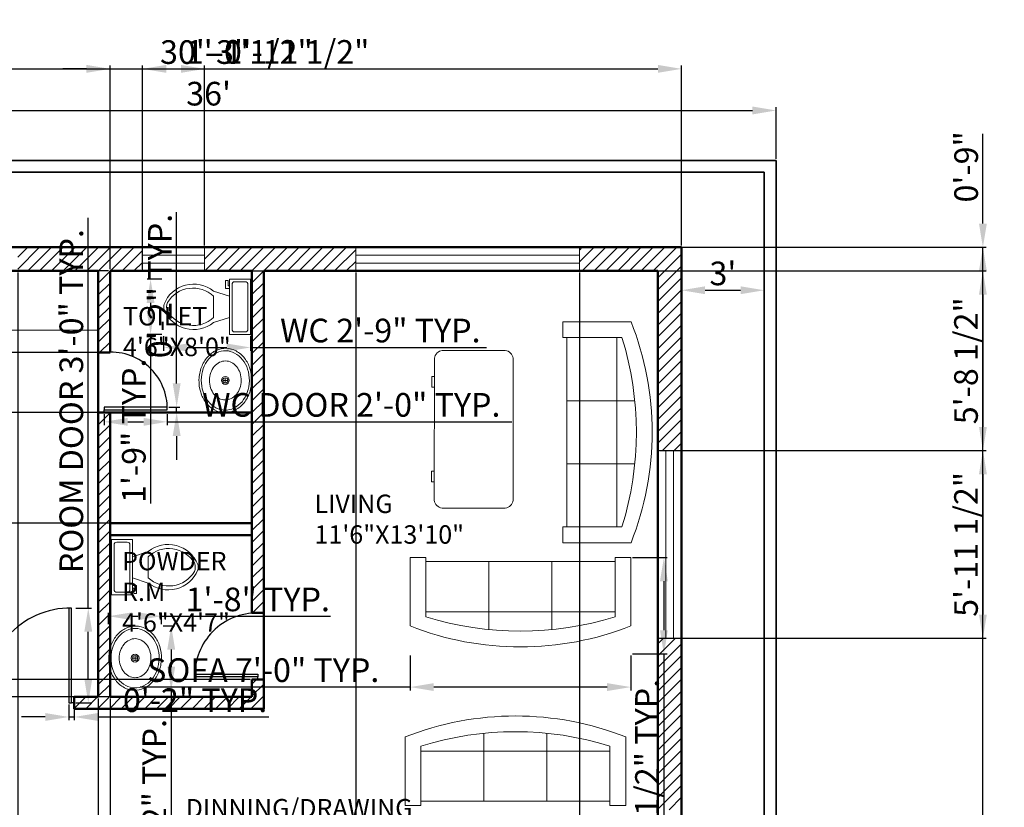
# Model space of a CAD drawing. Units: inches. Extents: x 53662 to 54269, y 37303 to 38048.
# Tile 6 of 6: x 53894 to 54269, y 37749 to 38048. Entities that reach past the tile are written whole.
import ezdxf

# ---------------------------------------------------------------- set-up
doc = ezdxf.new("R2010")
doc.units = ezdxf.units.IN
for name, color, linetype, lineweight in [('A-ANNO-DIMS', 2, 'Continuous', 18), ('A-AREA-IDEN', 7, 'Continuous', 25), ('A-DOOR', 3, 'Continuous', 25), ('A-FLOR-CASE', 8, 'Continuous', 18), ('A-FLOR-FIXT', 9, 'Continuous', 18), ('A-FURN', 8, 'Continuous', 18), ('A-GLAZ', 4, 'Continuous', 18), ('A-WALL', 7, 'Continuous', 50), ('C-PROP', 7, 'Continuous', 35)]:
    doc.layers.add(name, color=color, linetype=linetype, lineweight=lineweight)
doc.layers.add('A-WALL-PATT', color=244, linetype='Continuous', lineweight=13, true_color=0x991b1e)
doc.styles.get("Standard").update_dxf_attribs({"font": 'arial.ttf'})
doc.dimstyles.new('ISO-25', dxfattribs={"dimtxt": 9, "dimasz": 9, "dimexe": 1.25, "dimexo": 0.625, "dimtad": 1, "dimdec": 1, "dimrnd": 9, "dimlunit": 3, "dimtxsty": 'Standard', "dimcen": 2.5, "dimadec": 0, "dimazin": 0, "dimtfac": 1, "dimtdec": 1, "dimtmove": 0, "dimatfit": 3, "dimfxl": 1, "dimarcsym": 0})

# ---------------------------------------------------------------- blocks, each defined once
blk = doc.blocks.new('Toilet - top')
for p, q in [((9.5, -6), (9.5, -2)), ((-10, -8.5), (-8, -8.5)), ((-10, -9.5), (-10, -8.5)), ((-7, -9.5), (-10, -9.5)), ((-8, -8.5), (-8, -8)), ((-7, -8), (-7, -9.5)), ((-4, -8), (-6, -14)), ((4, -8), (6, -14)), ((4, -14), (-4, -14))]:
    blk.add_line(p, q)
blk.add_lwpolyline([(10.5, -8), (10.5, 0), (-10.5, 0), (-10.5, -8)], close=True)
for points in [[(-9.5, -2), (-9.5, -6)], [(8.5, -1), (-8.5, -1)], [(-8.5, -7), (8.5, -7)]]:
    blk.add_lwpolyline(points)
for centre, radius, start, end in [((-8.62, -1.88), 0.884, 81.8699, 188.1301), ((8.62, -1.88), 0.884, 351.8699, 98.1301), ((-8.62, -6.12), 0.884, 171.8699, 278.1301), ((8.62, -6.12), 0.884, 261.8699, 8.1301), ((3.52, -21.58), 12.17, 141.4691, 247.9714), ((4.2, -21.82), 11.33, 136.3677, 238.9468), ((-3.52, -21.58), 12.17, 292.0284, 38.5307), ((-4.2, -21.82), 11.33, 301.053, 43.6321), ((0, -27.88), 4, 245.7318, 294.2682), ((0, -29), 4, 254.8605, 285.1395)]:
    blk.add_arc(centre, radius, start, end)
blk = doc.blocks.new('Sink - Oval top')
for p, q in [((-1, 0), (1, 0)), ((0, 1), (0, -1))]:
    blk.add_line(p, q)
for points in [[(-12.23, 0.39, 0.117634), (-11.46, -3.36, 0.104469), (-8.88, -6.8, 0.090016), (-5.08, -9.07, 0.08192), (-0.32, -10.02, 0.08192), (4.49, -9.38, 0.090016), (8.42, -7.36, 0.104469), (11.22, -4.09, 0.117634), (12.23, -0.39, 0.117634), (11.46, 3.36, 0.104469), (8.88, 6.8, 0.090016), (5.08, 9.07, 0.08192), (0.32, 10.02, 0.08192), (-4.49, 9.38, 0.090016), (-8.42, 7.36, 0.104469), (-11.22, 4.09, 0.117634)], [(-11.29, 0.16, 0.118622), (-10.52, -3.25, 0.104678), (-8.07, -6.36, 0.089562), (-4.54, -8.37, 0.081185), (-0.13, -9.15, 0.081185), (4.3, -8.49, 0.089562), (7.89, -6.58, 0.104678), (10.42, -3.55, 0.118622), (11.29, -0.16, 0.118622), (10.52, 3.25, 0.104678), (8.07, 6.36, 0.089562), (4.54, 8.37, 0.081185), (0.13, 9.15, 0.081185), (-4.3, 8.49, 0.089562), (-7.89, 6.58, 0.104678), (-10.42, 3.55, 0.118622)], [(-7.42, 0.08, 0.118283), (-6.91, -2.17, 0.104607), (-5.29, -4.21, 0.089718), (-2.97, -5.53, 0.081436), (-0.07, -6.04, 0.081436), (2.84, -5.59, 0.089718), (5.2, -4.33, 0.104607), (6.86, -2.32, 0.118283), (7.42, -0.08, 0.118283), (6.91, 2.17, 0.104607), (5.29, 4.21, 0.089718), (2.97, 5.53, 0.081436), (0.07, 6.04, 0.081436), (-2.84, 5.59, 0.089718), (-5.2, 4.33, 0.104607), (-6.86, 2.32, 0.118283)]]:
    blk.add_lwpolyline(points, format="xyb", close=True)
for radius in [1.5, 1]:
    blk.add_circle((0, 0), radius)
blk = doc.blocks.new('Sofa - Roundback 7 ft.')
for p, q in [((-12.00002, -32.4421), (-12.00003, -6.5971)), ((11.99997, -32.4421), (11.99998, -6.5971)), ((-36.000027, -34), (-36.000027, -11.4696)), ((-35.999844, -13.3819), (35.9998, -13.3819)), ((35.99998, -34), (35.99998, -11.4696)), ((-36.000027, -32.4421), (35.99998, -32.4421))]:
    blk.add_line(p, q)
for points in [[(-36.000027, -34), (-42.000027, -34), (-42.000027, -8)], [(41.99998, -8), (41.99998, -34), (35.99998, -34)]]:
    blk.add_lwpolyline(points)
for centre, radius, start, end in [((0, -114.25), 114.25, 68.43141, 111.5686), ((-0.00001, -127.1968), 121.1968, 72.72033, 107.2797)]:
    blk.add_arc(centre, radius, start, end)
blk = doc.blocks.new('Desk - 30 x 60 in.')
for p, q in [((-26.999995, 0), (26.999995, 0)), ((-29.999995, -27), (-29.999995, -3)), ((29.999995, -3), (29.999995, -27)), ((26.999995, -30), (-26.999995, -30)), ((-20.000005, -30), (-20.000005, -31)), ((-20.000005, -31), (-16.000005, -31)), ((-16.000005, -31), (-16.000005, -30)), ((15.999995, -31), (15.999995, -30)), ((19.999995, -31), (15.999995, -31)), ((19.999995, -30), (19.999995, -31))]:
    blk.add_line(p, q)
for centre, start, end in [((-26.499995, -3.5), 98.1301, 171.8699), ((26.499995, -3.5), 8.130102, 81.8699), ((-26.499995, -26.5), 188.1301, 261.8699), ((26.499995, -26.5), 278.1301, 351.8699)]:
    blk.add_arc(centre, 3.535534, start, end)
blk = doc.blocks.new('*D11')
at = {"layer": 'A-ANNO-DIMS', "color": 0, "lineweight": -2, "transparency": 16777216}
for p, q in [((54146.11, 37961.24), (54146.11, 37944.26)), ((54177.61, 37961.24), (54177.61, 37944.26)), ((54155.11, 37945.51), (54168.61, 37945.51))]:
    blk.add_line(p, q, dxfattribs=at)
at = {"layer": 'A-ANNO-DIMS', "color": 0, "transparency": 16777216}
for points in [[(54155.11, 37947.01), (54155.11, 37944.01), (54146.11, 37945.51)], [(54168.61, 37947.01), (54168.61, 37944.01), (54177.61, 37945.51)]]:
    blk.add_solid(points, dxfattribs=at)
at = {"layer": 'Defpoints', "color": 0, "transparency": 16777216}
for p in [(54146.11, 37961.86), (54177.61, 37961.86), (54177.61, 37945.51)]:
    blk.add_point(p, dxfattribs=at)
at = {"layer": 'A-ANNO-DIMS', "color": 0, "transparency": 16777216, "insert": (54161.86, 37950.74), "char_height": 9, "attachment_point": 5}
blk.add_mtext("3'", dxfattribs=at)
blk = doc.blocks.new('*D14')
at = {"layer": 'A-ANNO-DIMS', "color": 0, "lineweight": -2, "transparency": 16777216}
for p, q in [((53750.11, 37995.49), (53750.11, 38015.14)), ((54182.11, 37995.49), (54182.11, 38015.14)), ((53759.11, 38013.89), (54173.11, 38013.89))]:
    blk.add_line(p, q, dxfattribs=at)
at = {"layer": 'A-ANNO-DIMS', "color": 0, "transparency": 16777216}
for points in [[(53759.11, 38015.39), (53759.11, 38012.39), (53750.11, 38013.89)], [(54173.11, 38015.39), (54173.11, 38012.39), (54182.11, 38013.89)]]:
    blk.add_solid(points, dxfattribs=at)
at = {"layer": 'Defpoints', "color": 0, "transparency": 16777216}
for p in [(54182.11, 38013.89), (53750.11, 37994.86), (54182.11, 37994.86)]:
    blk.add_point(p, dxfattribs=at)
at = {"layer": 'A-ANNO-DIMS', "color": 0, "transparency": 16777216, "insert": (53966.11, 38019.11), "char_height": 9, "attachment_point": 5}
blk.add_mtext("36'", dxfattribs=at)
blk = doc.blocks.new('DOOR-LEAF-36IN')
for p, q in [((1, 36), (0, 36)), ((0, 36), (0, 0)), ((1, 0), (1, 36)), ((0, 0), (1, 0)), ((2, 0), (1, 0))]:
    blk.add_line(p, q)
blk = doc.blocks.new('DOOR-LEAF-24IN')
for p, q in [((24, 2), (0, 2)), ((0, 2), (0, 1)), ((0, 0), (0, 1)), ((0, 1), (24, 1)), ((24, 1), (24, 2))]:
    blk.add_line(p, q)
blk = doc.blocks.new('*D30')
at = {"layer": 'A-ANNO-DIMS', "color": 0, "lineweight": -2, "transparency": 16777216}
for p, q in [((54042.81, 37806.54), (54042.81, 37793.32)), ((54126.81, 37806.54), (54126.81, 37793.32)), ((54042.81, 37794.57), (53940.02, 37794.57)), ((54117.81, 37794.57), (54051.81, 37794.57))]:
    blk.add_line(p, q, dxfattribs=at)
at = {"layer": 'A-ANNO-DIMS', "color": 0, "transparency": 16777216}
for points in [[(54051.81, 37796.07), (54051.81, 37793.07), (54042.81, 37794.57)], [(54117.81, 37796.07), (54117.81, 37793.07), (54126.81, 37794.57)]]:
    blk.add_solid(points, dxfattribs=at)
at = {"layer": 'Defpoints', "color": 0, "transparency": 16777216}
for p in [(54042.81, 37807.17), (54126.81, 37807.17), (54042.81, 37794.57)]:
    blk.add_point(p, dxfattribs=at)
at = {"layer": 'A-ANNO-DIMS', "color": 0, "transparency": 16777216, "insert": (53986.91, 37799.85), "char_height": 9, "attachment_point": 5}
blk.add_mtext('SOFA 7\'-0" TYP.', dxfattribs=at)
blk = doc.blocks.new('*D31')
at = {"layer": 'A-ANNO-DIMS', "color": 0, "lineweight": -2, "transparency": 16777216}
for p, q in [((54127.43, 37843.84), (54140.66, 37843.84)), ((54139.41, 37834.84), (54139.41, 37816.17)), ((54127.43, 37807.17), (54140.66, 37807.17)), ((54139.41, 37807.17), (54139.41, 37721.1))]:
    blk.add_line(p, q, dxfattribs=at)
at = {"layer": 'A-ANNO-DIMS', "color": 0, "transparency": 16777216}
for points in [[(54137.91, 37834.84), (54140.91, 37834.84), (54139.41, 37843.84)], [(54137.91, 37816.17), (54140.91, 37816.17), (54139.41, 37807.17)]]:
    blk.add_solid(points, dxfattribs=at)
at = {"layer": 'Defpoints', "color": 0, "transparency": 16777216}
for p in [(54126.81, 37843.84), (54126.81, 37807.17), (54139.41, 37807.17)]:
    blk.add_point(p, dxfattribs=at)
at = {"layer": 'A-ANNO-DIMS', "color": 0, "transparency": 16777216, "insert": (54134.13, 37759.63), "char_height": 9, "attachment_point": 5, "rotation": 90}
blk.add_mtext('3\'-0 1/2" TYP.', dxfattribs=at)
blk = doc.blocks.new('*D36')
at = {"layer": 'A-ANNO-DIMS', "color": 0, "lineweight": -2, "transparency": 16777216}
for p, q in [((53948.99, 37928.07), (53948.99, 37922.49)), ((53982.03, 37928.07), (53982.03, 37922.49)), ((53957.99, 37923.74), (53973.03, 37923.74)), ((53982.03, 37923.74), (54071.95, 37923.74))]:
    blk.add_line(p, q, dxfattribs=at)
at = {"layer": 'A-ANNO-DIMS', "color": 0, "transparency": 16777216}
for points in [[(53957.99, 37925.24), (53957.99, 37922.24), (53948.99, 37923.74)], [(53973.03, 37925.24), (53973.03, 37922.24), (53982.03, 37923.74)]]:
    blk.add_solid(points, dxfattribs=at)
at = {"layer": 'Defpoints', "color": 0, "transparency": 16777216}
for p in [(53948.99, 37928.7), (53982.03, 37928.7), (53982.03, 37923.74)]:
    blk.add_point(p, dxfattribs=at)
at = {"layer": 'A-ANNO-DIMS', "color": 0, "transparency": 16777216, "insert": (54031.49, 37929.02), "char_height": 9, "attachment_point": 5}
blk.add_mtext('WC 2\'-9" TYP.', dxfattribs=at)
blk = doc.blocks.new('*D37')
at = {"layer": 'A-ANNO-DIMS', "color": 0, "lineweight": -2, "transparency": 16777216}
for p, q in [((53948.36, 37949.7), (53942.78, 37949.7)), ((53944.03, 37940.7), (53944.03, 37937.7)), ((53948.36, 37928.7), (53942.78, 37928.7)), ((53944.03, 37928.7), (53944.03, 37864.43))]:
    blk.add_line(p, q, dxfattribs=at)
at = {"layer": 'A-ANNO-DIMS', "color": 0, "transparency": 16777216}
for points in [[(53942.53, 37940.7), (53945.53, 37940.7), (53944.03, 37949.7)], [(53942.53, 37937.7), (53945.53, 37937.7), (53944.03, 37928.7)]]:
    blk.add_solid(points, dxfattribs=at)
at = {"layer": 'Defpoints', "color": 0, "transparency": 16777216}
for p in [(53948.99, 37949.7), (53944.03, 37928.7), (53948.99, 37928.7)]:
    blk.add_point(p, dxfattribs=at)
at = {"layer": 'A-ANNO-DIMS', "color": 0, "transparency": 16777216, "insert": (53938.81, 37892.06), "char_height": 9, "attachment_point": 5, "rotation": 90}
blk.add_mtext('1\'-9" TYP.', dxfattribs=at)
blk = doc.blocks.new('*D38')
at = {"layer": 'A-ANNO-DIMS', "color": 0, "lineweight": -2, "transparency": 16777216}
for p, q in [((53948.84, 37817.85), (53953.14, 37817.85)), ((53951.89, 37808.85), (53951.89, 37802.3)), ((53948.84, 37793.3), (53953.14, 37793.3)), ((53951.89, 37793.3), (53951.89, 37666.39))]:
    blk.add_line(p, q, dxfattribs=at)
at = {"layer": 'A-ANNO-DIMS', "color": 0, "transparency": 16777216}
for points in [[(53950.39, 37808.85), (53953.39, 37808.85), (53951.89, 37817.85)], [(53950.39, 37802.3), (53953.39, 37802.3), (53951.89, 37793.3)]]:
    blk.add_solid(points, dxfattribs=at)
at = {"layer": 'Defpoints', "color": 0, "transparency": 16777216}
for p in [(53948.21, 37817.85), (53948.21, 37793.3), (53951.89, 37793.3)]:
    blk.add_point(p, dxfattribs=at)
at = {"layer": 'A-ANNO-DIMS', "color": 0, "transparency": 16777216, "insert": (53946.62, 37725.34), "char_height": 9, "attachment_point": 5, "rotation": 90}
blk.add_mtext('BASIN 2\'-0 1/2" TYP.', dxfattribs=at)
blk = doc.blocks.new('*D39')
at = {"layer": 'A-ANNO-DIMS', "color": 0, "lineweight": -2, "transparency": 16777216}
for p, q in [((53928.07, 37818.47), (53928.07, 37822.78)), ((53937.07, 37821.53), (53939.21, 37821.53)), ((53948.21, 37818.47), (53948.21, 37822.78)), ((53948.21, 37821.53), (54012.47, 37821.53))]:
    blk.add_line(p, q, dxfattribs=at)
at = {"layer": 'A-ANNO-DIMS', "color": 0, "transparency": 16777216}
for points in [[(53937.07, 37823.03), (53937.07, 37820.03), (53928.07, 37821.53)], [(53939.21, 37823.03), (53939.21, 37820.03), (53948.21, 37821.53)]]:
    blk.add_solid(points, dxfattribs=at)
at = {"layer": 'Defpoints', "color": 0, "transparency": 16777216}
for p in [(53948.21, 37821.53), (53928.07, 37817.85), (53948.21, 37817.85)]:
    blk.add_point(p, dxfattribs=at)
at = {"layer": 'A-ANNO-DIMS', "color": 0, "transparency": 16777216, "insert": (53984.84, 37826.75), "char_height": 9, "attachment_point": 5}
blk.add_mtext('1\'-8" TYP.', dxfattribs=at)
blk = doc.blocks.new('*D40')
at = {"layer": 'A-ANNO-DIMS', "color": 0, "lineweight": -2, "transparency": 16777216}
for p, q in [((53920.32, 37824.61), (53920.32, 37973.07)), ((53915.54, 37824.61), (53921.57, 37824.61)), ((53920.32, 37797.61), (53920.32, 37815.61)), ((53915.54, 37788.61), (53921.57, 37788.61))]:
    blk.add_line(p, q, dxfattribs=at)
at = {"layer": 'A-ANNO-DIMS', "color": 0, "transparency": 16777216}
for points in [[(53918.82, 37815.61), (53921.82, 37815.61), (53920.32, 37824.61)], [(53918.82, 37797.61), (53921.82, 37797.61), (53920.32, 37788.61)]]:
    blk.add_solid(points, dxfattribs=at)
at = {"layer": 'Defpoints', "color": 0, "transparency": 16777216}
for p in [(53914.92, 37824.61), (53920.32, 37824.61), (53914.92, 37788.61)]:
    blk.add_point(p, dxfattribs=at)
at = {"layer": 'A-ANNO-DIMS', "color": 0, "transparency": 16777216, "insert": (53915.03, 37903.34), "char_height": 9, "attachment_point": 5, "rotation": 90}
blk.add_mtext('ROOM DOOR 3\'-0" TYP.', dxfattribs=at)
blk = doc.blocks.new('*D41')
at = {"layer": 'A-ANNO-DIMS', "color": 0, "lineweight": -2, "transparency": 16777216}
for p, q in [((53912.92, 37787.99), (53912.92, 37781.96)), ((53914.92, 37787.99), (53914.92, 37781.96)), ((53903.92, 37783.21), (53894.92, 37783.21)), ((53912.92, 37783.21), (53914.92, 37783.21)), ((53923.92, 37783.21), (53989.03, 37783.21))]:
    blk.add_line(p, q, dxfattribs=at)
at = {"layer": 'A-ANNO-DIMS', "color": 0, "transparency": 16777216}
for points in [[(53903.92, 37784.71), (53903.92, 37781.71), (53912.92, 37783.21)], [(53923.92, 37784.71), (53923.92, 37781.71), (53914.92, 37783.21)]]:
    blk.add_solid(points, dxfattribs=at)
at = {"layer": 'Defpoints', "color": 0, "transparency": 16777216}
for p in [(53912.92, 37788.61), (53914.92, 37788.61), (53914.92, 37783.21)]:
    blk.add_point(p, dxfattribs=at)
at = {"layer": 'A-ANNO-DIMS', "color": 0, "transparency": 16777216, "insert": (53960.97, 37788.43), "char_height": 9, "attachment_point": 5}
blk.add_mtext('0\'-2" TYP.', dxfattribs=at)
blk = doc.blocks.new('*D42')
at = {"layer": 'A-ANNO-DIMS', "color": 0, "lineweight": -2, "transparency": 16777216}
for p, q in [((53926.36, 37898.44), (53926.36, 37894.21)), ((53950.36, 37898.44), (53950.36, 37894.21)), ((53935.36, 37895.46), (53941.36, 37895.46)), ((53950.36, 37895.46), (54081.49, 37895.46))]:
    blk.add_line(p, q, dxfattribs=at)
at = {"layer": 'A-ANNO-DIMS', "color": 0, "transparency": 16777216}
for points in [[(53935.36, 37896.96), (53935.36, 37893.96), (53926.36, 37895.46)], [(53941.36, 37896.96), (53941.36, 37893.96), (53950.36, 37895.46)]]:
    blk.add_solid(points, dxfattribs=at)
at = {"layer": 'Defpoints', "color": 0, "transparency": 16777216}
for p in [(53926.36, 37899.06), (53950.36, 37899.06), (53950.36, 37895.46)]:
    blk.add_point(p, dxfattribs=at)
at = {"layer": 'A-ANNO-DIMS', "color": 0, "transparency": 16777216, "insert": (54020.43, 37900.75), "char_height": 9, "attachment_point": 5}
blk.add_mtext('WC DOOR 2\'-0" TYP.', dxfattribs=at)
blk = doc.blocks.new('*D43')
at = {"layer": 'A-ANNO-DIMS', "color": 0, "lineweight": -2, "transparency": 16777216}
for p, q in [((53953.96, 37910.06), (53953.96, 37975.17)), ((53950.99, 37901.06), (53955.21, 37901.06)), ((53950.99, 37899.06), (53955.21, 37899.06)), ((53953.96, 37899.06), (53953.96, 37901.06)), ((53953.96, 37890.06), (53953.96, 37881.06))]:
    blk.add_line(p, q, dxfattribs=at)
at = {"layer": 'A-ANNO-DIMS', "color": 0, "transparency": 16777216}
for points in [[(53952.46, 37910.06), (53955.46, 37910.06), (53953.96, 37901.06)], [(53952.46, 37890.06), (53955.46, 37890.06), (53953.96, 37899.06)]]:
    blk.add_solid(points, dxfattribs=at)
at = {"layer": 'Defpoints', "color": 0, "transparency": 16777216}
for p in [(53950.36, 37901.06), (53950.36, 37899.06), (53953.96, 37901.06)]:
    blk.add_point(p, dxfattribs=at)
at = {"layer": 'A-ANNO-DIMS', "color": 0, "transparency": 16777216, "insert": (53948.74, 37947.12), "char_height": 9, "attachment_point": 5, "rotation": 90}
blk.add_mtext('0\'-2" TYP.', dxfattribs=at)
blk = doc.blocks.new('*D50')
at = {"layer": 'A-ANNO-DIMS', "color": 0, "lineweight": -2, "transparency": 16777216}
for p, q in [((53783.11, 37962.49), (53783.11, 38030.96)), ((53792.11, 38029.71), (54137.11, 38029.71)), ((54146.11, 37962.49), (54146.11, 38030.96))]:
    blk.add_line(p, q, dxfattribs=at)
at = {"layer": 'A-ANNO-DIMS', "color": 0, "transparency": 16777216}
for points in [[(53792.11, 38031.21), (53792.11, 38028.21), (53783.11, 38029.71)], [(54137.11, 38031.21), (54137.11, 38028.21), (54146.11, 38029.71)]]:
    blk.add_solid(points, dxfattribs=at)
at = {"layer": 'Defpoints', "color": 0, "transparency": 16777216}
for p in [(54146.11, 38029.71), (53783.11, 37961.86), (54146.11, 37961.86)]:
    blk.add_point(p, dxfattribs=at)
at = {"layer": 'A-ANNO-DIMS', "color": 0, "transparency": 16777216, "insert": (53964.61, 38034.93), "char_height": 9, "attachment_point": 5}
blk.add_mtext('30\'-3"', dxfattribs=at)
blk = doc.blocks.new('*D51')
at = {"layer": 'A-ANNO-DIMS', "color": 0, "lineweight": -2, "transparency": 16777216}
for p, q in [((54146.74, 37961.86), (54262.07, 37961.86)), ((54260.82, 37471.86), (54260.82, 37952.86)), ((53987.74, 37462.86), (54262.07, 37462.86))]:
    blk.add_line(p, q, dxfattribs=at)
at = {"layer": 'A-ANNO-DIMS', "color": 0, "transparency": 16777216}
for points in [[(54259.32, 37952.86), (54262.32, 37952.86), (54260.82, 37961.86)], [(54259.32, 37471.86), (54262.32, 37471.86), (54260.82, 37462.86)]]:
    blk.add_solid(points, dxfattribs=at)
at = {"layer": 'Defpoints', "color": 0, "transparency": 16777216}
for p in [(54146.11, 37961.86), (54260.82, 37961.86), (53987.11, 37462.86)]:
    blk.add_point(p, dxfattribs=at)
at = {"layer": 'A-ANNO-DIMS', "color": 0, "transparency": 16777216, "insert": (54255.68, 37712.36), "char_height": 9, "attachment_point": 5, "rotation": 90}
blk.add_mtext('41\'-7"', dxfattribs=at)
blk = doc.blocks.new('*D55')
at = {"layer": 'A-ANNO-DIMS', "color": 0, "lineweight": -2, "transparency": 16777216}
for p, q in [((53849.2, 37952.24), (53849.2, 37309.49)), ((53893.52, 37952.24), (53893.52, 37309.49)), ((53858.2, 37310.74), (53884.52, 37310.74)), ((53893.52, 37310.74), (53948.66, 37310.74))]:
    blk.add_line(p, q, dxfattribs=at)
at = {"layer": 'A-ANNO-DIMS', "color": 0, "transparency": 16777216}
for points in [[(53858.2, 37312.24), (53858.2, 37309.24), (53849.2, 37310.74)], [(53884.52, 37312.24), (53884.52, 37309.24), (53893.52, 37310.74)]]:
    blk.add_solid(points, dxfattribs=at)
at = {"layer": 'Defpoints', "color": 0, "transparency": 16777216}
for p in [(53849.2, 37952.86), (53893.52, 37952.86), (53893.52, 37310.74)]:
    blk.add_point(p, dxfattribs=at)
at = {"layer": 'A-ANNO-DIMS', "color": 0, "transparency": 16777216, "insert": (53925.59, 37316.02), "char_height": 9, "attachment_point": 5}
blk.add_mtext('3\'-8 1/2"', dxfattribs=at)
blk = doc.blocks.new('*D56')
at = {"layer": 'A-ANNO-DIMS', "color": 0, "lineweight": -2, "transparency": 16777216}
for p, q in [((53919.61, 38029.71), (53910.61, 38029.71)), ((53928.61, 37953.49), (53928.61, 38030.96)), ((53928.61, 38029.71), (53940.97, 38029.71)), ((53940.97, 37953.49), (53940.97, 38030.96)), ((53949.97, 38029.71), (54004.27, 38029.71))]:
    blk.add_line(p, q, dxfattribs=at)
at = {"layer": 'A-ANNO-DIMS', "color": 0, "transparency": 16777216}
for points in [[(53919.61, 38031.21), (53919.61, 38028.21), (53928.61, 38029.71)], [(53949.97, 38031.21), (53949.97, 38028.21), (53940.97, 38029.71)]]:
    blk.add_solid(points, dxfattribs=at)
at = {"layer": 'Defpoints', "color": 0, "transparency": 16777216}
for p in [(53940.97, 38029.71), (53928.61, 37952.86), (53940.97, 37952.86)]:
    blk.add_point(p, dxfattribs=at)
at = {"layer": 'A-ANNO-DIMS', "color": 0, "transparency": 16777216, "insert": (53981.62, 38034.99), "char_height": 9, "attachment_point": 5}
blk.add_mtext('1\'-0 1/2"', dxfattribs=at)
blk = doc.blocks.new('*D57')
at = {"layer": 'A-ANNO-DIMS', "color": 0, "lineweight": -2, "transparency": 16777216}
for p, q in [((53940.97, 37962.49), (53940.97, 38030.96)), ((53949.97, 38029.71), (53955.61, 38029.71)), ((53964.61, 37962.49), (53964.61, 38030.96)), ((53964.61, 38029.71), (54025.91, 38029.71))]:
    blk.add_line(p, q, dxfattribs=at)
at = {"layer": 'A-ANNO-DIMS', "color": 0, "transparency": 16777216}
for points in [[(53949.97, 38031.21), (53949.97, 38028.21), (53940.97, 38029.71)], [(53955.61, 38031.21), (53955.61, 38028.21), (53964.61, 38029.71)]]:
    blk.add_solid(points, dxfattribs=at)
at = {"layer": 'Defpoints', "color": 0, "transparency": 16777216}
for p in [(53964.61, 38029.71), (53940.97, 37961.86), (53964.61, 37961.86)]:
    blk.add_point(p, dxfattribs=at)
at = {"layer": 'A-ANNO-DIMS', "color": 0, "transparency": 16777216, "insert": (53999.76, 38034.99), "char_height": 9, "attachment_point": 5}
blk.add_mtext('1\'-11 1/2"', dxfattribs=at)
blk = doc.blocks.new('*D58')
at = {"layer": 'A-ANNO-DIMS', "color": 0, "lineweight": -2, "transparency": 16777216}
for p, q in [((54022.12, 37952.24), (54022.12, 37309.49)), ((54107.27, 37952.24), (54107.27, 37309.49)), ((54031.12, 37310.74), (54098.27, 37310.74))]:
    blk.add_line(p, q, dxfattribs=at)
at = {"layer": 'A-ANNO-DIMS', "color": 0, "transparency": 16777216}
for points in [[(54031.12, 37312.24), (54031.12, 37309.24), (54022.12, 37310.74)], [(54098.27, 37312.24), (54098.27, 37309.24), (54107.27, 37310.74)]]:
    blk.add_solid(points, dxfattribs=at)
at = {"layer": 'Defpoints', "color": 0, "transparency": 16777216}
for p in [(54022.12, 37952.86), (54107.27, 37952.86), (54107.27, 37310.74)]:
    blk.add_point(p, dxfattribs=at)
at = {"layer": 'A-ANNO-DIMS', "color": 0, "transparency": 16777216, "insert": (54064.7, 37315.88), "char_height": 9, "attachment_point": 5}
blk.add_mtext('7\'-1"', dxfattribs=at)
blk = doc.blocks.new('*D59')
at = {"layer": 'A-ANNO-DIMS', "color": 0, "lineweight": -2, "transparency": 16777216}
for p, q in [((54107.27, 37952.24), (54107.27, 37309.49)), ((54137.11, 37952.24), (54137.11, 37309.49)), ((54116.27, 37310.74), (54128.11, 37310.74))]:
    blk.add_line(p, q, dxfattribs=at)
at = {"layer": 'A-ANNO-DIMS', "color": 0, "transparency": 16777216}
for points in [[(54116.27, 37312.24), (54116.27, 37309.24), (54107.27, 37310.74)], [(54128.11, 37312.24), (54128.11, 37309.24), (54137.11, 37310.74)]]:
    blk.add_solid(points, dxfattribs=at)
at = {"layer": 'Defpoints', "color": 0, "transparency": 16777216}
for p in [(54107.27, 37952.86), (54137.11, 37952.86), (54137.11, 37310.74)]:
    blk.add_point(p, dxfattribs=at)
at = {"layer": 'A-ANNO-DIMS', "color": 0, "transparency": 16777216, "insert": (54122.19, 37315.96), "char_height": 9, "attachment_point": 5}
blk.add_mtext('2\'-6"', dxfattribs=at)
blk = doc.blocks.new('*D60')
at = {"layer": 'A-ANNO-DIMS', "color": 0, "lineweight": -2, "transparency": 16777216}
for p, q in [((53924.11, 37790.24), (53924.11, 37309.49)), ((53928.61, 37790.24), (53928.61, 37309.49)), ((53915.11, 37310.74), (53906.11, 37310.74)), ((53924.11, 37310.74), (53928.61, 37310.74)), ((53937.61, 37310.74), (53992.76, 37310.74))]:
    blk.add_line(p, q, dxfattribs=at)
at = {"layer": 'A-ANNO-DIMS', "color": 0, "transparency": 16777216}
for points in [[(53915.11, 37312.24), (53915.11, 37309.24), (53924.11, 37310.74)], [(53937.61, 37312.24), (53937.61, 37309.24), (53928.61, 37310.74)]]:
    blk.add_solid(points, dxfattribs=at)
at = {"layer": 'Defpoints', "color": 0, "transparency": 16777216}
for p in [(53924.11, 37790.86), (53928.61, 37790.86), (53928.61, 37310.74)]:
    blk.add_point(p, dxfattribs=at)
at = {"layer": 'A-ANNO-DIMS', "color": 0, "transparency": 16777216, "insert": (53969.69, 37316.02), "char_height": 9, "attachment_point": 5}
blk.add_mtext('0\'-4 1/2"', dxfattribs=at)
blk = doc.blocks.new('*D61')
at = {"layer": 'A-ANNO-DIMS', "color": 0, "lineweight": -2, "transparency": 16777216}
for p, q in [((54260.82, 37970.86), (54260.82, 38005.03)), ((53965.24, 37961.86), (54262.07, 37961.86)), ((54260.82, 37952.86), (54260.82, 37961.86)), ((53965.24, 37952.86), (54262.07, 37952.86)), ((54260.82, 37943.86), (54260.82, 37934.86))]:
    blk.add_line(p, q, dxfattribs=at)
at = {"layer": 'A-ANNO-DIMS', "color": 0, "transparency": 16777216}
for points in [[(54259.32, 37970.86), (54262.32, 37970.86), (54260.82, 37961.86)], [(54259.32, 37943.86), (54262.32, 37943.86), (54260.82, 37952.86)]]:
    blk.add_solid(points, dxfattribs=at)
at = {"layer": 'Defpoints', "color": 0, "transparency": 16777216}
for p in [(53964.61, 37961.86), (54260.82, 37961.86), (53964.61, 37952.86)]:
    blk.add_point(p, dxfattribs=at)
at = {"layer": 'A-ANNO-DIMS', "color": 0, "transparency": 16777216, "insert": (54255.6, 37992.45), "char_height": 9, "attachment_point": 5, "rotation": 90}
blk.add_mtext('0\'-9"', dxfattribs=at)
blk = doc.blocks.new('*D66')
at = {"layer": 'A-ANNO-DIMS', "color": 0, "lineweight": -2, "transparency": 16777216}
for p, q in [((54137.74, 37952.86), (54262.07, 37952.86)), ((54260.82, 37943.86), (54260.82, 37893.55)), ((54137.74, 37884.55), (54262.07, 37884.55))]:
    blk.add_line(p, q, dxfattribs=at)
at = {"layer": 'A-ANNO-DIMS', "color": 0, "transparency": 16777216}
for points in [[(54259.32, 37943.86), (54262.32, 37943.86), (54260.82, 37952.86)], [(54259.32, 37893.55), (54262.32, 37893.55), (54260.82, 37884.55)]]:
    blk.add_solid(points, dxfattribs=at)
at = {"layer": 'Defpoints', "color": 0, "transparency": 16777216}
for p in [(54137.11, 37952.86), (54137.11, 37884.55), (54260.82, 37884.55)]:
    blk.add_point(p, dxfattribs=at)
at = {"layer": 'A-ANNO-DIMS', "color": 0, "transparency": 16777216, "insert": (54255.55, 37918.7), "char_height": 9, "attachment_point": 5, "rotation": 90}
blk.add_mtext('5\'-8 1/2"', dxfattribs=at)
blk = doc.blocks.new('*D67')
at = {"layer": 'A-ANNO-DIMS', "color": 0, "lineweight": -2, "transparency": 16777216}
for p, q in [((54137.74, 37884.55), (54262.07, 37884.55)), ((54260.82, 37875.55), (54260.82, 37822.18)), ((54137.74, 37813.18), (54262.07, 37813.18))]:
    blk.add_line(p, q, dxfattribs=at)
at = {"layer": 'A-ANNO-DIMS', "color": 0, "transparency": 16777216}
for points in [[(54259.32, 37875.55), (54262.32, 37875.55), (54260.82, 37884.55)], [(54259.32, 37822.18), (54262.32, 37822.18), (54260.82, 37813.18)]]:
    blk.add_solid(points, dxfattribs=at)
at = {"layer": 'Defpoints', "color": 0, "transparency": 16777216}
for p in [(54137.11, 37884.55), (54137.11, 37813.18), (54260.82, 37813.18)]:
    blk.add_point(p, dxfattribs=at)
at = {"layer": 'A-ANNO-DIMS', "color": 0, "transparency": 16777216, "insert": (54255.55, 37848.86), "char_height": 9, "attachment_point": 5, "rotation": 90}
blk.add_mtext('5\'-11 1/2"', dxfattribs=at)
blk = doc.blocks.new('*D72')
at = {"layer": 'A-ANNO-DIMS', "color": 0, "lineweight": -2, "transparency": 16777216}
for p, q in [((53981.99, 37899.06), (53679.5, 37899.06)), ((53680.75, 37865.86), (53680.75, 37890.06)), ((53981.99, 37856.86), (53679.5, 37856.86))]:
    blk.add_line(p, q, dxfattribs=at)
at = {"layer": 'A-ANNO-DIMS', "color": 0, "transparency": 16777216}
for points in [[(53679.25, 37890.06), (53682.25, 37890.06), (53680.75, 37899.06)], [(53679.25, 37865.86), (53682.25, 37865.86), (53680.75, 37856.86)]]:
    blk.add_solid(points, dxfattribs=at)
at = {"layer": 'Defpoints', "color": 0, "transparency": 16777216}
for p in [(53680.75, 37899.06), (53982.61, 37899.06), (53982.61, 37856.86)]:
    blk.add_point(p, dxfattribs=at)
at = {"layer": 'A-ANNO-DIMS', "color": 0, "transparency": 16777216, "insert": (53675.53, 37877.96), "char_height": 9, "attachment_point": 5, "rotation": 90}
blk.add_mtext('3\'-6"', dxfattribs=at)
blk = doc.blocks.new('*D73')
at = {"layer": 'A-ANNO-DIMS', "color": 0, "lineweight": -2, "transparency": 16777216}
for p, q in [((53927.99, 37952.86), (53679.5, 37952.86)), ((53680.75, 37930.83), (53680.75, 37943.86)), ((53927.99, 37921.83), (53679.5, 37921.83))]:
    blk.add_line(p, q, dxfattribs=at)
at = {"layer": 'A-ANNO-DIMS', "color": 0, "transparency": 16777216}
for points in [[(53679.25, 37943.86), (53682.25, 37943.86), (53680.75, 37952.86)], [(53679.25, 37930.83), (53682.25, 37930.83), (53680.75, 37921.83)]]:
    blk.add_solid(points, dxfattribs=at)
at = {"layer": 'Defpoints', "color": 0, "transparency": 16777216}
for p in [(53680.75, 37952.86), (53928.61, 37952.86), (53928.61, 37921.83)]:
    blk.add_point(p, dxfattribs=at)
at = {"layer": 'A-ANNO-DIMS', "color": 0, "transparency": 16777216, "insert": (53675.61, 37937.35), "char_height": 9, "attachment_point": 5, "rotation": 90}
blk.add_mtext('2\'-7"', dxfattribs=at)
blk = doc.blocks.new('*D74')
at = {"layer": 'A-ANNO-DIMS', "color": 0, "lineweight": -2, "transparency": 16777216}
for p, q in [((53680.75, 37806.48), (53680.75, 37861.62)), ((53981.99, 37797.48), (53679.5, 37797.48)), ((53680.75, 37790.86), (53680.75, 37797.48)), ((53981.99, 37790.86), (53679.5, 37790.86)), ((53680.75, 37781.86), (53680.75, 37772.86))]:
    blk.add_line(p, q, dxfattribs=at)
at = {"layer": 'A-ANNO-DIMS', "color": 0, "transparency": 16777216}
for points in [[(53679.25, 37806.48), (53682.25, 37806.48), (53680.75, 37797.48)], [(53679.25, 37781.86), (53682.25, 37781.86), (53680.75, 37790.86)]]:
    blk.add_solid(points, dxfattribs=at)
at = {"layer": 'Defpoints', "color": 0, "transparency": 16777216}
for p in [(53680.75, 37797.48), (53982.61, 37797.48), (53982.61, 37790.86)]:
    blk.add_point(p, dxfattribs=at)
at = {"layer": 'A-ANNO-DIMS', "color": 0, "transparency": 16777216, "insert": (53675.47, 37838.55), "char_height": 9, "attachment_point": 5, "rotation": 90}
blk.add_mtext('0\'-6 1/2"', dxfattribs=at)

msp = doc.modelspace()

# ---------------------------------------------------------------- hatches: boundary and pattern name
at = {"layer": 'A-WALL-PATT'}
h = msp.add_hatch(dxfattribs=at)
h.set_pattern_fill('ANSI31', color=256)
h.paths.add_polyline_path([(53792.11, 37952.86), (53849.2, 37952.86), (53849.2, 37961.86), (53783.11, 37961.86), (53783.11, 37861.42), (53792.11, 37861.42)])
h.paths.add_polyline_path([(53940.97, 37961.86), (53893.52, 37961.86), (53893.52, 37952.86), (53924.11, 37952.86), (53924.11, 37921.83), (53926.36, 37921.83, -0.026334), (53928.61, 37921.99), (53928.61, 37930.37), (53928.61, 37952.86), (53940.97, 37952.86)])
h.paths.add_polyline_path([(53792.11, 37786.36), (53882.05, 37786.36), (53882.05, 37788.61, -0.017862), (53881.82, 37790.86), (53792.11, 37790.86), (53792.11, 37806.76), (53783.11, 37806.76), (53783.11, 37732.86), (53792.11, 37732.86)])
h.paths.add_polyline_path([(53792.11, 37672.86), (53783.11, 37672.86), (53783.11, 37615.86), (53804.11, 37615.86), (53804.11, 37599.43), (53813.11, 37599.43), (53813.11, 37620.36), (53922.61, 37620.36), (53922.61, 37624.86), (53792.11, 37624.86)])
h.paths.add_polyline_path([(53978.11, 37572.86), (53927.11, 37572.86), (53927.11, 37620.36), (53922.61, 37620.36), (53922.61, 37568.36), (53978.11, 37568.36)])
h.paths.add_polyline_path([(53927.11, 37624.86), (53922.61, 37624.86), (53922.61, 37620.36), (53927.11, 37620.36)])
h.paths.add_polyline_path([(53987.11, 37615.86), (54079.03, 37615.86), (54079.03, 37624.86), (53978.11, 37624.86), (53978.11, 37471.86), (53926.17, 37471.86), (53926.17, 37462.86), (53987.11, 37462.86)])
h.paths.add_polyline_path([(53813.11, 37561.58), (53804.11, 37561.58), (53804.11, 37471.86), (53783.11, 37471.86), (53783.11, 37462.86), (53873.85, 37462.86), (53873.85, 37471.86), (53813.11, 37471.86)])
h.paths.add_polyline_path([(54146.11, 37687.42), (54137.11, 37687.42), (54137.11, 37624.86), (54128.99, 37624.86), (54128.99, 37615.86), (54146.11, 37615.86)])
h.paths.add_polyline_path([(54146.11, 37813.18), (54137.11, 37813.18), (54137.11, 37747.89), (54146.11, 37747.89)])
h.paths.add_polyline_path([(54146.11, 37961.86), (54107.27, 37961.86), (54107.27, 37952.86), (54137.11, 37952.86), (54137.11, 37884.55), (54146.11, 37884.55)])
h.paths.add_polyline_path([(54022.12, 37961.86), (53964.61, 37961.86), (53964.61, 37952.86), (53982.61, 37952.86), (53982.61, 37822.8), (53987.11, 37822.8), (53987.11, 37952.86), (54022.12, 37952.86)])
h.paths.add_polyline_path([(53928.61, 37899.06), (53924.11, 37899.06), (53924.11, 37790.86), (53914.92, 37790.86), (53914.92, 37786.36), (53987.11, 37786.36), (53987.11, 37797.48), (53982.61, 37797.48), (53982.61, 37790.86), (53928.61, 37790.86), (53928.61, 37801.6, -0.072813), (53928.13, 37805.9, -0.05664), (53928.61, 37809.23)])

# ---------------------------------------------------------------- linework, layer by layer
at = {"layer": 'A-DOOR'}
for centre, radius, start, end in [((53928.95, 37900.56), 21.42, 358.6628, 96.9187), ((53913.42, 37792.95), 31.67, 89.0952, 187.8757), ((53984.68, 37798.98), 23.82, 89.5613, 181.2026)]:
    msp.add_arc(centre, radius, start, end, dxfattribs=at)
at = {"layer": 'A-FLOR-CASE'}
msp.add_line((53924.11, 37930.37), (53792.11, 37930.37), dxfattribs=at)
at = {"layer": 'A-GLAZ'}
for p, q in [((53940.97, 37961.86), (53940.97, 37952.86)), ((53940.97, 37958.86), (53964.61, 37958.86)), ((53964.61, 37961.86), (53964.61, 37952.86)), ((54022.12, 37961.86), (54022.12, 37952.86)), ((54022.12, 37958.86), (54107.27, 37958.86)), ((54107.27, 37961.86), (54107.27, 37952.86)), ((53940.97, 37955.86), (53964.61, 37955.86)), ((54022.12, 37955.86), (54107.27, 37955.86)), ((54146.11, 37884.55), (54137.11, 37884.55)), ((54140.11, 37813.18), (54140.11, 37884.55)), ((54143.11, 37813.18), (54143.11, 37884.55)), ((54146.11, 37813.18), (54137.11, 37813.18))]:
    msp.add_line(p, q, dxfattribs=at)
at = {"layer": 'A-WALL'}
for p, q in [((54146.11, 37961.86), (53783.11, 37961.86)), ((54146.11, 37615.86), (54146.11, 37961.86)), ((53924.11, 37952.86), (53792.11, 37952.86)), ((53924.11, 37952.86), (53924.11, 37790.86)), ((53928.61, 37952.86), (53928.61, 37930.37)), ((53982.61, 37952.86), (53928.61, 37952.86)), ((53982.61, 37952.86), (53982.61, 37822.8)), ((54137.11, 37952.86), (53987.11, 37952.86)), ((53987.11, 37952.86), (53987.11, 37786.36)), ((54137.11, 37624.86), (54137.11, 37952.86)), ((53928.61, 37930.37), (53928.61, 37921.83)), ((53928.61, 37921.83), (53924.11, 37921.83)), ((53928.61, 37899.06), (53924.11, 37899.06)), ((53928.61, 37899.06), (53982.61, 37899.06)), ((53928.61, 37899.06), (53928.61, 37790.86)), ((53982.61, 37856.86), (53928.61, 37856.86)), ((53982.61, 37852.36), (53928.61, 37852.36)), ((53987.11, 37822.8), (53982.61, 37822.8)), ((53987.11, 37797.48), (53982.61, 37797.48)), ((53982.61, 37797.48), (53982.61, 37790.86)), ((53924.11, 37790.86), (53914.92, 37790.86)), ((53914.92, 37790.86), (53914.92, 37786.36)), ((53982.61, 37790.86), (53928.61, 37790.86)), ((53987.11, 37786.36), (53914.92, 37786.36))]:
    msp.add_line(p, q, dxfattribs=at)
at = {"layer": 'C-PROP'}
for p, q in [((54182.11, 37994.86), (53750.11, 37994.86)), ((54182.11, 37418.86), (54182.11, 37994.86)), ((54177.61, 37990.36), (53754.61, 37990.36)), ((54177.61, 37442.85), (54177.61, 37990.36))]:
    msp.add_line(p, q, dxfattribs=at)

# ---------------------------------------------------------------- block references
at = {"layer": 'A-DOOR'}
for name, p in [('DOOR-LEAF-24IN', (53926.36, 37899.06)), ('DOOR-LEAF-36IN', (53912.92, 37788.61))]:
    msp.add_blockref(name, p, dxfattribs=at)
at = {"layer": 'A-DOOR', "extrusion": (0, 0, -1), "zscale": -1}
msp.add_blockref('DOOR-LEAF-24IN', (-53984.86, 37797.47), dxfattribs=at)
at = {"layer": 'A-FLOR-FIXT'}
for name, p, rotation in [('Toilet - top', (53982.03, 37939.2), 270), ('Sink - Oval top', (53972.48, 37911.2), 270), ('Toilet - top', (53929.17, 37840.16), 89.99999999999999), ('Sink - Oval top', (53938.14, 37805.57), 270)]:
    msp.add_blockref(name, p, dxfattribs=dict(at, rotation=rotation))
at = {"layer": 'A-FURN'}
for name, p, rotation in [('Sofa - Roundback 7 ft.', (54134.92, 37891.5), 270), ('Desk - 30 x 60 in.', (54082.03, 37892.63), 269.9533541638235), ('Sofa - Roundback 7 ft.', (54084.81, 37809.84), 180)]:
    msp.add_blockref(name, p, dxfattribs=dict(at, rotation=rotation))
msp.add_blockref('Sofa - Roundback 7 ft.', (54082.89, 37783.59), dxfattribs=at)

# ---------------------------------------------------------------- texts
at = {"layer": 'A-AREA-IDEN', "char_height": 7, "attachment_point": 1}
for s, width, insert in [('TOILET\\P4\'6"X8\'0"', 40.1945, (53933.52, 37939.11)), ('LIVING \\P11\'6"X13\'10"', 84.2154, (54006.41, 37867.78)), ('POWDER\\PR.M\\P4\'6"X4\'7"', 40.1945, (53933.17, 37845.99)), ('DINNING/DRAWING\\P21\'9"X12\'0"', 148.2626, (53957.4, 37752.01))]:
    msp.add_mtext_dynamic_manual_height_columns(s, width=width, gutter_width=12.5, heights=[0], dxfattribs=dict(at, insert=insert))

# ---------------------------------------------------------------- dimensions: what is measured, and where the dimension line sits
at = {"layer": 'A-ANNO-DIMS'}
for base, p1, p2, override, picture, middle in [((53940.97, 38029.71), (53928.61, 37952.86), (53940.97, 37952.86), {"dimdec": 1, "dimlfac": 1, "dimrnd": 0, "dimzin": 1, "dimdsep": 46, "dimlunit": 4, "dimfrac": 2}, '*D56', (53981.62, 38034.99)), ((53964.61, 38029.71), (53940.97, 37961.86), (53964.61, 37961.86), {"dimdec": 1, "dimlfac": 1, "dimrnd": 0, "dimzin": 1, "dimdsep": 46, "dimlunit": 4, "dimfrac": 2}, '*D57', (53999.76, 38034.99)), ((54146.11, 38029.71), (53783.11, 37961.86), (54146.11, 37961.86), {"dimdec": 1, "dimlfac": 1, "dimrnd": 0, "dimzin": 1, "dimdsep": 46, "dimlunit": 4, "dimfrac": 2}, '*D50', (53964.61, 38034.93)), ((54182.11, 38013.89), (53750.11, 37994.86), (54182.11, 37994.86), {"dimclrd": 0, "dimclre": 0, "dimclrt": 0}, '*D14', (53966.11, 38019.11)), ((54177.61, 37945.51), (54146.11, 37961.86), (54177.61, 37961.86), {"dimclrd": 0, "dimclre": 0, "dimclrt": 0}, '*D11', (54161.86, 37950.74)), ((53893.52, 37310.74), (53849.2, 37952.86), (53893.52, 37952.86), {"dimdec": 1, "dimlfac": 1, "dimrnd": 0, "dimzin": 1, "dimdsep": 46, "dimlunit": 4, "dimfrac": 2}, '*D55', (53925.59, 37316.02)), ((54107.2677, 37310.7389), (54022.1239, 37952.8602), (54107.2677, 37952.8602), {"dimdec": 1, "dimlfac": 1, "dimrnd": 0, "dimzin": 1, "dimdsep": 46, "dimlunit": 4, "dimfrac": 2}, '*D58', (54064.6958, 37315.8823)), ((54137.11, 37310.74), (54107.27, 37952.86), (54137.11, 37952.86), {"dimdec": 1, "dimlfac": 1, "dimrnd": 0, "dimzin": 1, "dimdsep": 46, "dimlunit": 4, "dimfrac": 2}, '*D59', (54122.19, 37315.96)), ((53928.61, 37310.74), (53924.11, 37790.86), (53928.61, 37790.86), {"dimdec": 1, "dimlfac": 1, "dimrnd": 0, "dimzin": 1, "dimdsep": 46, "dimlunit": 4, "dimfrac": 2}, '*D60', (53969.69, 37316.02))]:
    dim = msp.add_linear_dim(base=base, p1=p1, p2=p2, dimstyle='ISO-25', override=override, dxfattribs=at)
    dim.commit()
    dim.dimension.update_dxf_attribs({"geometry": picture, "text_midpoint": middle})
for base, p1, p2, picture, middle in [((54260.82, 37961.86), (53964.61, 37952.86), (53964.61, 37961.86), '*D61', (54255.6, 37992.45)), ((54260.82, 37961.86), (53987.11, 37462.86), (54146.11, 37961.86), '*D51', (54255.68, 37712.36)), ((53680.75, 37952.86), (53928.61, 37921.83), (53928.61, 37952.86), '*D73', (53675.61, 37937.35)), ((54260.82, 37884.55), (54137.11, 37952.86), (54137.11, 37884.55), '*D66', (54255.55, 37918.7)), ((53680.75, 37899.06), (53982.61, 37856.86), (53982.61, 37899.06), '*D72', (53675.53, 37877.96)), ((54260.82, 37813.18), (54137.11, 37884.55), (54137.11, 37813.18), '*D67', (54255.55, 37848.86)), ((53680.75, 37797.48), (53982.61, 37790.86), (53982.61, 37797.48), '*D74', (53675.47, 37838.55))]:
    dim = msp.add_linear_dim(base=base, p1=p1, p2=p2, angle=90, dimstyle='ISO-25', override={"dimdec": 1, "dimlfac": 1, "dimrnd": 0, "dimzin": 1, "dimdsep": 46, "dimlunit": 4, "dimfrac": 2}, dxfattribs=at)
    dim.commit()
    dim.dimension.update_dxf_attribs({"geometry": picture, "text_midpoint": middle})
for base, p1, p2, angle, text, picture, middle in [((53953.96, 37901.06), (53950.36, 37899.06), (53950.36, 37901.06), 90, '<> TYP.', '*D43', (53948.74, 37947.12)), ((53920.32, 37824.61), (53914.92, 37788.61), (53914.92, 37824.61), 90, 'ROOM DOOR <> TYP.', '*D40', (53915.03, 37903.34)), ((53944.03, 37928.7), (53948.99, 37949.7), (53948.99, 37928.7), 270, '<> TYP.', '*D37', (53938.81, 37892.06)), ((54139.41, 37807.17), (54126.81, 37843.84), (54126.81, 37807.17), 270, '<> TYP.', '*D31', (54134.13, 37759.63)), ((54042.81, 37794.57), (54126.81, 37807.17), (54042.81, 37807.17), 180, 'SOFA <> TYP.', '*D30', (53986.91, 37799.85)), ((53951.894, 37793.2972), (53948.2113, 37817.8481), (53948.2113, 37793.2972), 270, 'BASIN <> TYP.', '*D38', (53946.6155, 37725.3441))]:
    dim = msp.add_linear_dim(base=base, p1=p1, p2=p2, angle=angle, text=text, dimstyle='ISO-25', override={"dimdec": 1, "dimlfac": 1, "dimrnd": 0, "dimzin": 1, "dimdsep": 46, "dimlunit": 4, "dimfrac": 2}, dxfattribs=at)
    dim.commit()
    dim.dimension.update_dxf_attribs({"geometry": picture, "text_midpoint": middle})
for base, p1, p2, text, picture, middle in [((53982.03, 37923.74), (53948.99, 37928.7), (53982.03, 37928.7), 'WC <> TYP.', '*D36', (54031.49, 37929.02)), ((53950.36, 37895.46), (53926.36, 37899.06), (53950.36, 37899.06), 'WC DOOR <> TYP.', '*D42', (54020.43, 37900.75)), ((53948.21, 37821.53), (53928.07, 37817.85), (53948.21, 37817.85), '<> TYP.', '*D39', (53984.84, 37826.75)), ((53914.92, 37783.21), (53912.92, 37788.61), (53914.92, 37788.61), '<> TYP.', '*D41', (53960.97, 37788.43))]:
    dim = msp.add_linear_dim(base=base, p1=p1, p2=p2, text=text, dimstyle='ISO-25', override={"dimdec": 1, "dimlfac": 1, "dimrnd": 0, "dimzin": 1, "dimdsep": 46, "dimlunit": 4, "dimfrac": 2}, dxfattribs=at)
    dim.commit()
    dim.dimension.update_dxf_attribs({"geometry": picture, "text_midpoint": middle})

doc.saveas('drawing.dxf')
